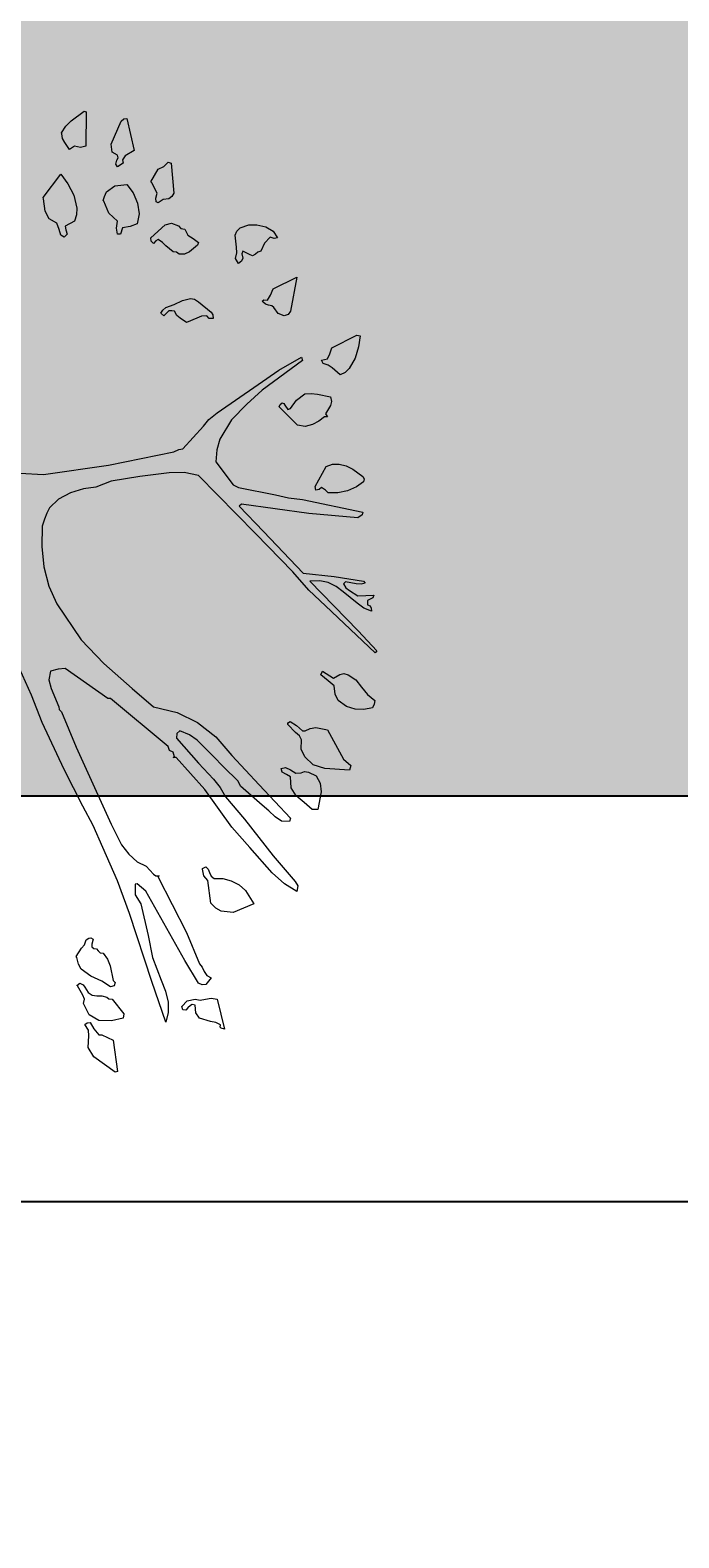
# Model space of a CAD drawing. Units: inches. Extents: x 84 to 1044, y -280 to 906.
# Tile 42 of 105: x 941 to 955, y -129 to -96. Entities that reach past the tile are written whole.
import ezdxf

# ---------------------------------------------------------------- set-up
doc = ezdxf.new("R2010")
doc.units = ezdxf.units.IN
for name, color, linetype, lineweight in [('A-ANNO-DIMS', 2, 'Continuous', 18), ('C-PROP', 7, 'Continuous', 25), ('L-PLNT', 114, 'Continuous', 15)]:
    doc.layers.add(name, color=color, linetype=linetype, lineweight=lineweight)
doc.layers.add('L-PLNT-PATT', color=9, linetype='Continuous', lineweight=9, true_color=0xafd9aa)
doc.styles.get("Standard").update_dxf_attribs({"font": 'arial.ttf'})
doc.dimstyles.get("Standard").update_dxf_attribs({"dimtxt": 0.18, "dimasz": 0.18, "dimexe": 0.18, "dimexo": 0.0625, "dimgap": 0.09, "dimtad": 0, "dimtih": 1, "dimtoh": 1, "dimdec": 4, "dimzin": 0, "dimdsep": 46, "dimtxsty": 'Standard', "dimcen": 0.09, "dimadec": 0, "dimazin": 0, "dimtfac": 1, "dimtdec": 4, "dimtofl": 0, "dimtmove": 0, "dimatfit": 3, "dimfxl": 1, "dimtolj": 1, "dimtzin": 0, "dimarcsym": 0})

# ---------------------------------------------------------------- blocks, each defined once
blk = doc.blocks.new('A$C37E508DF')
for p, q in [((0.9605, 1.4257), (0.9686, 1.4334)), ((0.9686, 1.4334), (0.9875, 1.4476)), ((0.9875, 1.4476), (0.9905, 1.4467)), ((0.9905, 1.4467), (0.9896, 1.3966)), ((1.0269, 1.3996), (1.0411, 1.433)), ((1.0411, 1.433), (1.045, 1.4365)), ((1.045, 1.4365), (1.0497, 1.4369)), ((1.0497, 1.4369), (1.0604, 1.3901)), ((0.9545, 1.4159), (0.9605, 1.4257)), ((0.9549, 1.4146), (0.9545, 1.4159)), ((0.9558, 1.4077), (0.9549, 1.4146)), ((0.9592, 1.4017), (0.9558, 1.4077)), ((0.966, 1.3914), (0.9592, 1.4017)), ((0.9703, 1.3944), (0.966, 1.3914)), ((0.9733, 1.3966), (0.9703, 1.3944)), ((0.9819, 1.3944), (0.9733, 1.3966)), ((0.9896, 1.3966), (0.9819, 1.3944)), ((1.0282, 1.3876), (1.0269, 1.3996)), ((1.0359, 1.3833), (1.0282, 1.3876)), ((1.0604, 1.3901), (1.0471, 1.3824)), ((1.0334, 1.37), (1.0351, 1.376)), ((1.0359, 1.3661), (1.0334, 1.37)), ((1.0351, 1.376), (1.0368, 1.3794)), ((1.0368, 1.3794), (1.0359, 1.3833)), ((1.0441, 1.3717), (1.0359, 1.3661)), ((1.0471, 1.3824), (1.0432, 1.3764)), ((1.0432, 1.3764), (1.0441, 1.3717)), ((1.0955, 1.3631), (1.1033, 1.367)), ((1.1033, 1.367), (1.1097, 1.373)), ((1.1097, 1.373), (1.114, 1.3717)), ((1.114, 1.3717), (1.1183, 1.328)), ((0.9274, 1.3215), (0.9532, 1.3554)), ((0.9532, 1.3554), (0.9635, 1.3413)), ((1.0848, 1.3443), (1.0955, 1.3631)), ((1.0861, 1.343), (1.0848, 1.3443)), ((1.0938, 1.328), (1.0861, 1.343)), ((0.9279, 1.3194), (0.9274, 1.3215)), ((0.9635, 1.3413), (0.9721, 1.325)), ((0.9721, 1.325), (0.9768, 1.3061)), ((1.0149, 1.3172), (1.0171, 1.3232)), ((1.0171, 1.3232), (1.0197, 1.3297)), ((1.0197, 1.3297), (1.0321, 1.3387)), ((1.0321, 1.3387), (1.0497, 1.3404)), ((1.0497, 1.3404), (1.0587, 1.3284)), ((1.0587, 1.3284), (1.0651, 1.3134)), ((1.0917, 1.3207), (1.0938, 1.328)), ((1.0925, 1.3151), (1.0917, 1.3207)), ((1.1153, 1.3228), (1.111, 1.3194)), ((1.1183, 1.328), (1.1153, 1.3228)), ((0.9305, 1.3018), (0.9279, 1.3194)), ((0.9365, 1.2902), (0.9305, 1.3018)), ((0.9768, 1.3061), (0.9763, 1.2962)), ((1.0162, 1.3164), (1.0149, 1.3172)), ((1.0231, 1.2988), (1.0162, 1.3164)), ((1.0359, 1.2868), (1.0231, 1.2988)), ((1.0651, 1.3134), (1.0677, 1.2975)), ((1.0955, 1.3138), (1.0925, 1.3151)), ((1.1028, 1.3185), (1.0955, 1.3138)), ((1.111, 1.3194), (1.1028, 1.3185)), ((0.9476, 1.2842), (0.9365, 1.2902)), ((0.951, 1.2748), (0.9476, 1.2842)), ((0.9733, 1.2868), (0.9596, 1.2799)), ((0.9596, 1.2799), (0.9605, 1.2744)), ((0.9763, 1.2962), (0.9733, 1.2868)), ((1.0347, 1.2769), (1.0359, 1.2868)), ((1.0359, 1.2679), (1.0347, 1.2769)), ((1.0432, 1.2774), (1.0402, 1.2679)), ((1.0544, 1.2791), (1.0432, 1.2774)), ((1.0647, 1.2829), (1.0544, 1.2791)), ((1.0677, 1.2975), (1.0647, 1.2829)), ((1.0848, 1.2628), (1.1054, 1.2817)), ((1.1054, 1.2817), (1.1148, 1.2842)), ((1.1148, 1.2842), (1.1247, 1.2804)), ((1.1247, 1.2804), (1.1281, 1.2765)), ((1.1281, 1.2765), (1.1341, 1.2752)), ((1.21, 1.2726), (1.2147, 1.2774)), ((1.2147, 1.2774), (1.2276, 1.2817)), ((1.2276, 1.2817), (1.2392, 1.2817)), ((1.2392, 1.2817), (1.2521, 1.2787)), ((1.2521, 1.2787), (1.2632, 1.2722)), ((0.9532, 1.2666), (0.951, 1.2748)), ((0.9583, 1.2636), (0.9532, 1.2666)), ((0.9626, 1.2679), (0.9583, 1.2636)), ((0.9605, 1.2744), (0.9626, 1.2679)), ((1.0402, 1.2679), (1.0359, 1.2679)), ((1.0852, 1.2576), (1.0848, 1.2628)), ((1.0883, 1.2546), (1.0852, 1.2576)), ((1.0921, 1.2585), (1.0883, 1.2546)), ((1.0955, 1.2602), (1.0921, 1.2585)), ((1.1015, 1.2559), (1.0955, 1.2602)), ((1.1063, 1.2508), (1.1015, 1.2559)), ((1.1341, 1.2752), (1.1384, 1.2666)), ((1.1384, 1.2666), (1.1461, 1.2619)), ((1.1461, 1.2619), (1.1539, 1.2559)), ((1.1539, 1.2559), (1.1526, 1.2521)), ((1.2075, 1.2666), (1.21, 1.2726)), ((1.2096, 1.2491), (1.2075, 1.2666)), ((1.2503, 1.2551), (1.2448, 1.2431)), ((1.2585, 1.2636), (1.2503, 1.2551)), ((1.2645, 1.2615), (1.2585, 1.2636)), ((1.2632, 1.2722), (1.2692, 1.2628)), ((1.2692, 1.2628), (1.2645, 1.2615)), ((1.117, 1.2422), (1.1063, 1.2508)), ((1.1221, 1.2418), (1.117, 1.2422)), ((1.126, 1.2388), (1.1221, 1.2418)), ((1.1337, 1.2388), (1.126, 1.2388)), ((1.141, 1.2422), (1.1337, 1.2388)), ((1.1526, 1.2521), (1.141, 1.2422)), ((1.2079, 1.2323), (1.21, 1.2409)), ((1.2126, 1.2251), (1.2079, 1.2323)), ((1.21, 1.2409), (1.2096, 1.2491)), ((1.2186, 1.2332), (1.2169, 1.2285)), ((1.2186, 1.2431), (1.2173, 1.2392)), ((1.2173, 1.2392), (1.2186, 1.2332)), ((1.2285, 1.2383), (1.2186, 1.2431)), ((1.2328, 1.2366), (1.2285, 1.2383)), ((1.2371, 1.2388), (1.2328, 1.2366)), ((1.2405, 1.2418), (1.2371, 1.2388)), ((1.2448, 1.2431), (1.2405, 1.2418)), ((1.2169, 1.2285), (1.2126, 1.2251)), ((1.2589, 1.1792), (1.2628, 1.1882)), ((1.2628, 1.1882), (1.2975, 1.2053)), ((1.2975, 1.2053), (1.2885, 1.1556)), ((1.1187, 1.1655), (1.1307, 1.1714)), ((1.1307, 1.1714), (1.1423, 1.1744)), ((1.1423, 1.1744), (1.1483, 1.1732)), ((1.1483, 1.1732), (1.1539, 1.1693)), ((1.1539, 1.1693), (1.1727, 1.1543)), ((1.2469, 1.1702), (1.2495, 1.1723)), ((1.2478, 1.1693), (1.2469, 1.1702)), ((1.2516, 1.1659), (1.2478, 1.1693)), ((1.2495, 1.1723), (1.2546, 1.1719)), ((1.2546, 1.1719), (1.2589, 1.1792)), ((1.099, 1.153), (1.102, 1.1573)), ((1.1033, 1.1487), (1.099, 1.153)), ((1.102, 1.1573), (1.1063, 1.1612)), ((1.111, 1.156), (1.1033, 1.1487)), ((1.1063, 1.1612), (1.1187, 1.1655)), ((1.1153, 1.1564), (1.111, 1.156)), ((1.1191, 1.1556), (1.1153, 1.1564)), ((1.1226, 1.1492), (1.1191, 1.1556)), ((1.1273, 1.1453), (1.1226, 1.1492)), ((1.1367, 1.1393), (1.1273, 1.1453)), ((1.1517, 1.1453), (1.1367, 1.1393)), ((1.1586, 1.1483), (1.1517, 1.1453)), ((1.1663, 1.1487), (1.1586, 1.1483)), ((1.1697, 1.1449), (1.1663, 1.1487)), ((1.1757, 1.1449), (1.1697, 1.1449)), ((1.1727, 1.1543), (1.1749, 1.1504)), ((1.1749, 1.1504), (1.1757, 1.1449)), ((1.2563, 1.1646), (1.2516, 1.1659)), ((1.2611, 1.1637), (1.2563, 1.1646)), ((1.2641, 1.1612), (1.2611, 1.1637)), ((1.2701, 1.1522), (1.2641, 1.1612)), ((1.2791, 1.1487), (1.2701, 1.1522)), ((1.2851, 1.1509), (1.2791, 1.1487)), ((1.2885, 1.1556), (1.2851, 1.1509)), ((1.3455, 1.0934), (1.3485, 1.102)), ((1.3485, 1.102), (1.385, 1.1209)), ((1.3875, 1.1037), (1.3828, 1.087)), ((1.385, 1.1209), (1.3897, 1.1196)), ((1.3897, 1.1196), (1.3875, 1.1037)), ((1.3057, 1.0835), (1.2469, 1.0402)), ((1.2713, 1.0694), (1.3044, 1.0887)), ((1.3044, 1.0887), (1.3057, 1.0835)), ((1.3335, 1.0844), (1.3421, 1.0861)), ((1.3361, 1.0793), (1.3335, 1.0844)), ((1.3434, 1.0771), (1.3361, 1.0793)), ((1.3421, 1.0861), (1.3455, 1.0934)), ((1.3828, 1.087), (1.3738, 1.072)), ((1.2409, 1.0488), (1.2713, 1.0694)), ((1.349, 1.0728), (1.3434, 1.0771)), ((1.3605, 1.063), (1.349, 1.0728)), ((1.3678, 1.0664), (1.3605, 1.063)), ((1.3738, 1.072), (1.3678, 1.0664)), ((1.1813, 1.0072), (1.2409, 1.0488)), ((1.2469, 1.0402), (1.2246, 1.0201)), ((1.2971, 1.0257), (1.3091, 1.0351)), ((1.3091, 1.0351), (1.3185, 1.0355)), ((1.3185, 1.0355), (1.3275, 1.0347)), ((1.3275, 1.0347), (1.3468, 1.0308)), ((1.2246, 1.0201), (1.2023, 0.9969)), ((1.2718, 1.0162), (1.2731, 1.0197)), ((1.2984, 0.9892), (1.2718, 1.0162)), ((1.2731, 1.0197), (1.2761, 1.0218)), ((1.2761, 1.0218), (1.2786, 1.0209)), ((1.2786, 1.0209), (1.2799, 1.0184)), ((1.2799, 1.0184), (1.2842, 1.0124)), ((1.2842, 1.0124), (1.2885, 1.0136)), ((1.2885, 1.0136), (1.2971, 1.0257)), ((1.3468, 1.018), (1.3391, 1.0059)), ((1.3468, 1.0308), (1.3481, 1.0239)), ((1.3481, 1.0239), (1.3468, 1.018)), ((1.1612, 0.9879), (1.1693, 0.9974)), ((1.1693, 0.9974), (1.1813, 1.0072)), ((1.2023, 0.9969), (1.1852, 0.9691)), ((1.3202, 0.9901), (1.3095, 0.9875)), ((1.3297, 0.9952), (1.3202, 0.9901)), ((1.3378, 1.0016), (1.3297, 0.9952)), ((1.3421, 1.0016), (1.3378, 1.0016)), ((1.3391, 1.0059), (1.3421, 1.0016)), ((1.1311, 0.9549), (1.1612, 0.9879)), ((1.1852, 0.9691), (1.1809, 0.9532)), ((1.3095, 0.9875), (1.2984, 0.9892)), ((1.0227, 0.9309), (1.1183, 0.9506)), ((1.1183, 0.9506), (1.1256, 0.954)), ((1.1256, 0.954), (1.1311, 0.9549)), ((1.1809, 0.9532), (1.1796, 0.936)), ((0.9279, 0.9172), (1.0227, 0.9309)), ((1.1796, 0.936), (1.2049, 0.9022)), ((1.3241, 0.9), (1.3404, 0.9292)), ((1.3404, 0.9292), (1.3494, 0.9322)), ((1.3494, 0.9322), (1.3592, 0.9326)), ((1.3592, 0.9326), (1.3695, 0.93)), ((1.3695, 0.93), (1.3794, 0.9253)), ((1.3794, 0.9253), (1.394, 0.9146)), ((0.8936, 0.9193), (0.9279, 0.9172)), ((1.0269, 0.9077), (1.0042, 0.8987)), ((1.0685, 0.9142), (1.0269, 0.9077)), ((1.1114, 0.9198), (1.0685, 0.9142)), ((1.1333, 0.9202), (1.1114, 0.9198)), ((1.1543, 0.9159), (1.1333, 0.9202)), ((1.2371, 0.8314), (1.1543, 0.9159)), ((1.2049, 0.9022), (1.2126, 0.8983)), ((1.3948, 0.9065), (1.3846, 0.8992)), ((1.394, 0.9146), (1.3957, 0.9112)), ((1.3957, 0.9112), (1.3948, 0.9065)), ((0.9498, 0.8816), (0.9369, 0.8687)), ((0.9673, 0.8906), (0.9498, 0.8816)), ((0.9866, 0.8962), (0.9673, 0.8906)), ((1.0042, 0.8987), (0.9866, 0.8962)), ((1.2126, 0.8983), (1.2662, 0.8876)), ((1.2662, 0.8876), (1.2855, 0.8833)), ((1.2855, 0.8833), (1.3057, 0.8807)), ((1.3057, 0.8807), (1.394, 0.8623)), ((1.3254, 0.8944), (1.3241, 0.9)), ((1.3301, 0.8957), (1.3254, 0.8944)), ((1.3335, 0.8983), (1.3301, 0.8957)), ((1.3395, 0.8944), (1.3335, 0.8983)), ((1.3434, 0.8906), (1.3395, 0.8944)), ((1.3571, 0.8906), (1.3434, 0.8906)), ((1.3713, 0.8936), (1.3571, 0.8906)), ((1.3846, 0.8992), (1.3713, 0.8936)), ((0.933, 0.861), (0.9296, 0.852)), ((0.9369, 0.8687), (0.933, 0.861)), ((1.2169, 0.8743), (1.2135, 0.8713)), ((1.2135, 0.8713), (1.2491, 0.834)), ((1.3151, 0.8606), (1.2169, 0.8743)), ((1.3863, 0.8541), (1.3151, 0.8606)), ((1.3927, 0.8584), (1.3863, 0.8541)), ((1.394, 0.8623), (1.3927, 0.8584)), ((0.9262, 0.8421), (0.9257, 0.8121)), ((0.9296, 0.852), (0.9262, 0.8421)), ((1.2919, 0.7752), (1.2371, 0.8314)), ((1.2491, 0.834), (1.3069, 0.7735)), ((0.9257, 0.8121), (0.9287, 0.7825)), ((0.9287, 0.7825), (0.936, 0.7542)), ((1.3151, 0.7487), (1.2919, 0.7752)), ((1.3069, 0.7735), (1.352, 0.7684)), ((0.936, 0.7542), (0.9476, 0.7285)), ((1.3391, 0.7255), (1.3151, 0.7487)), ((1.3309, 0.7624), (1.3164, 0.7615)), ((1.3164, 0.7615), (1.3871, 0.6891)), ((1.3434, 0.7598), (1.3309, 0.7624)), ((1.355, 0.7538), (1.3434, 0.7598)), ((1.352, 0.7684), (1.3948, 0.7615)), ((1.3653, 0.7461), (1.355, 0.7538)), ((1.3687, 0.7607), (1.3657, 0.7577)), ((1.3657, 0.7577), (1.3691, 0.7521)), ((1.3841, 0.7577), (1.3687, 0.7607)), ((1.3691, 0.7521), (1.3743, 0.7482)), ((1.3743, 0.7482), (1.3863, 0.7405)), ((1.3914, 0.7572), (1.3841, 0.7577)), ((1.397, 0.759), (1.3914, 0.7572)), ((1.3948, 0.7615), (1.397, 0.759)), ((0.9476, 0.7285), (0.9828, 0.6762)), ((1.3854, 0.7294), (1.3653, 0.7461)), ((1.3953, 0.7221), (1.3854, 0.7294)), ((1.3863, 0.7405), (1.4099, 0.7414)), ((1.4086, 0.7375), (1.4004, 0.7337)), ((1.4004, 0.7337), (1.4004, 0.7272)), ((1.4004, 0.7272), (1.4047, 0.7255)), ((1.4099, 0.7414), (1.4086, 0.7375)), ((1.4116, 0.6569), (1.3391, 0.7255)), ((1.4064, 0.7178), (1.3953, 0.7221)), ((1.4047, 0.7255), (1.406, 0.7221)), ((1.406, 0.7221), (1.4064, 0.7178)), ((1.3871, 0.6891), (1.4141, 0.6599)), ((0.9828, 0.6762), (1.0162, 0.6415)), ((1.0162, 0.6415), (1.0574, 0.605)), ((1.4141, 0.6599), (1.4116, 0.6569)), ((0.9103, 0.5956), (0.8932, 0.6342)), ((0.9382, 0.6303), (0.936, 0.6179)), ((0.936, 0.6179), (0.939, 0.605)), ((0.9493, 0.6333), (0.9382, 0.6303)), ((0.9596, 0.6342), (0.9493, 0.6333)), ((1.0218, 0.5904), (0.9596, 0.6342)), ((1.3327, 0.6252), (1.3348, 0.6303)), ((1.343, 0.6162), (1.3327, 0.6252)), ((1.3348, 0.6303), (1.3511, 0.62)), ((1.352, 0.6089), (1.343, 0.6162)), ((1.3511, 0.62), (1.3601, 0.6256)), ((1.3601, 0.6256), (1.3661, 0.6269)), ((1.3661, 0.6269), (1.3725, 0.6252)), ((1.3725, 0.6252), (1.3837, 0.6175)), ((1.3837, 0.6175), (1.3918, 0.6072)), ((0.9262, 0.5557), (0.9103, 0.5956)), ((0.939, 0.605), (0.9506, 0.5784)), ((1.0574, 0.605), (1.0883, 0.5784)), ((1.3533, 0.5969), (1.352, 0.6089)), ((1.358, 0.5874), (1.3533, 0.5969)), ((1.3918, 0.6072), (1.4004, 0.5964)), ((1.4004, 0.5964), (1.4111, 0.5874)), ((0.9506, 0.5784), (0.951, 0.5746)), ((0.951, 0.5746), (0.9545, 0.5711)), ((1.0256, 0.5904), (1.0218, 0.5904)), ((1.1097, 0.5205), (1.0256, 0.5904)), ((1.0883, 0.5784), (1.123, 0.5703)), ((1.37, 0.5789), (1.358, 0.5874)), ((1.3824, 0.575), (1.37, 0.5789)), ((1.3953, 0.5746), (1.3824, 0.575)), ((1.4077, 0.5771), (1.3953, 0.5746)), ((1.4103, 0.5823), (1.4077, 0.5771)), ((1.4111, 0.5874), (1.4103, 0.5823)), ((0.9583, 0.4871), (0.9262, 0.5557)), ((0.9545, 0.5711), (0.9759, 0.5193)), ((1.123, 0.5703), (1.1526, 0.5557)), ((1.1526, 0.5557), (1.1792, 0.5347)), ((1.2842, 0.554), (1.2855, 0.5557)), ((1.2842, 0.5527), (1.2842, 0.554)), ((1.2958, 0.5407), (1.2842, 0.5527)), ((1.2855, 0.5557), (1.2876, 0.557)), ((1.2876, 0.557), (1.2971, 0.551)), ((1.2971, 0.551), (1.3057, 0.5433)), ((1.1226, 0.5394), (1.1221, 0.5325)), ((1.1221, 0.5325), (1.1539, 0.4961)), ((1.1268, 0.5433), (1.1226, 0.5394)), ((1.141, 0.5377), (1.1268, 0.5433)), ((1.1521, 0.5296), (1.141, 0.5377)), ((1.1706, 0.5111), (1.1521, 0.5296)), ((1.1792, 0.5347), (1.2027, 0.5072)), ((1.3014, 0.536), (1.2958, 0.5407)), ((1.3044, 0.53), (1.3014, 0.536)), ((1.3039, 0.5167), (1.3044, 0.53)), ((1.3057, 0.5433), (1.3099, 0.5433)), ((1.3099, 0.5433), (1.3172, 0.5467)), ((1.3172, 0.5467), (1.3254, 0.548)), ((1.3254, 0.548), (1.3421, 0.5446)), ((1.3421, 0.5446), (1.3657, 0.5021)), ((0.9759, 0.5193), (1.0269, 0.4069)), ((1.1118, 0.5145), (1.1097, 0.5205)), ((1.117, 0.5124), (1.1118, 0.5145)), ((1.1191, 0.5055), (1.117, 0.5124)), ((1.1955, 0.4858), (1.1706, 0.5111)), ((1.2027, 0.5072), (1.2426, 0.4644)), ((1.3091, 0.5055), (1.3039, 0.5167)), ((0.9853, 0.4335), (0.9583, 0.4871)), ((1.117, 0.5042), (1.1191, 0.5055)), ((1.1217, 0.5042), (1.117, 0.5042)), ((1.1633, 0.4575), (1.1217, 0.5042)), ((1.1539, 0.4961), (1.1762, 0.4729)), ((1.207, 0.4747), (1.1955, 0.4858)), ((1.2748, 0.4884), (1.2812, 0.4897)), ((1.2761, 0.4832), (1.2748, 0.4884)), ((1.2812, 0.4897), (1.2885, 0.4862)), ((1.2885, 0.4862), (1.2962, 0.4815)), ((1.3039, 0.482), (1.3087, 0.4841)), ((1.3087, 0.4841), (1.3147, 0.4832)), ((1.3215, 0.4935), (1.3091, 0.5055)), ((1.3382, 0.4884), (1.3215, 0.4935)), ((1.3743, 0.4858), (1.3382, 0.4884)), ((1.3657, 0.5021), (1.3764, 0.4927)), ((1.3764, 0.4927), (1.3743, 0.4858)), ((1.1762, 0.4729), (1.1856, 0.4605)), ((1.2122, 0.47), (1.207, 0.4747)), ((1.2156, 0.4627), (1.2122, 0.47)), ((1.2469, 0.4348), (1.2156, 0.4627)), ((1.2426, 0.4644), (1.2885, 0.4159)), ((1.2825, 0.4798), (1.2761, 0.4832)), ((1.2885, 0.4764), (1.2825, 0.4798)), ((1.2894, 0.4601), (1.2885, 0.4764)), ((1.2962, 0.4815), (1.3039, 0.482)), ((1.3147, 0.4832), (1.3258, 0.4777)), ((1.3258, 0.4777), (1.3318, 0.4669)), ((1.3318, 0.4669), (1.3331, 0.4545)), ((1.2027, 0.4026), (1.1633, 0.4575)), ((1.1856, 0.4605), (1.1933, 0.4468)), ((1.1933, 0.4468), (1.2212, 0.4146)), ((1.2967, 0.4485), (1.2894, 0.4601)), ((1.3082, 0.4386), (1.2967, 0.4485)), ((1.3331, 0.4545), (1.3284, 0.4284)), ((1.0003, 0.4052), (0.9853, 0.4335)), ((1.2568, 0.4266), (1.2469, 0.4348)), ((1.2658, 0.4176), (1.2568, 0.4266)), ((1.3198, 0.4284), (1.3082, 0.4386)), ((1.3284, 0.4284), (1.3198, 0.4284)), ((1.0145, 0.373), (1.0003, 0.4052)), ((1.0269, 0.4069), (1.0419, 0.3769)), ((1.2289, 0.373), (1.2027, 0.4026)), ((1.2212, 0.4146), (1.2628, 0.361)), ((1.2752, 0.4116), (1.2658, 0.4176)), ((1.2868, 0.4108), (1.2752, 0.4116)), ((1.2885, 0.4159), (1.2868, 0.4108)), ((1.0419, 0.3769), (1.0527, 0.3632)), ((1.0359, 0.3246), (1.0145, 0.373)), ((1.0527, 0.3632), (1.0647, 0.352)), ((1.0647, 0.352), (1.078, 0.346)), ((1.2615, 0.3362), (1.2289, 0.373)), ((1.2628, 0.361), (1.2949, 0.3233)), ((1.078, 0.346), (1.0883, 0.334)), ((1.0883, 0.334), (1.0921, 0.3319)), ((1.0921, 0.3319), (1.0968, 0.3319)), ((1.0968, 0.3319), (1.0947, 0.3306)), ((1.0947, 0.3306), (1.1367, 0.2491)), ((1.1599, 0.3426), (1.1646, 0.3447)), ((1.1599, 0.3413), (1.1599, 0.3426)), ((1.162, 0.3319), (1.1599, 0.3413)), ((1.1676, 0.325), (1.162, 0.3319)), ((1.1646, 0.3447), (1.168, 0.3417)), ((1.168, 0.3417), (1.1702, 0.3366)), ((1.1702, 0.3366), (1.1727, 0.3314)), ((1.1727, 0.3314), (1.177, 0.3276)), ((1.2795, 0.3199), (1.2615, 0.3362)), ((1.0535, 0.2766), (1.0359, 0.3246)), ((1.0647, 0.3199), (1.0617, 0.3194)), ((1.0617, 0.3194), (1.0617, 0.304)), ((1.0711, 0.3147), (1.0647, 0.3199)), ((1.0775, 0.3092), (1.0711, 0.3147)), ((1.1341, 0.2084), (1.0775, 0.3092)), ((1.1719, 0.292), (1.1676, 0.325)), ((1.177, 0.3276), (1.1895, 0.3276)), ((1.1895, 0.3276), (1.2019, 0.3246)), ((1.2019, 0.3246), (1.2135, 0.3186)), ((1.2135, 0.3186), (1.2225, 0.3104)), ((1.2225, 0.3104), (1.2349, 0.2911)), ((1.2975, 0.3087), (1.2795, 0.3199)), ((1.2949, 0.3233), (1.2988, 0.3173)), ((1.2988, 0.3173), (1.2975, 0.3087)), ((1.0617, 0.304), (1.0698, 0.2911)), ((1.0698, 0.2911), (1.0805, 0.2448)), ((1.1792, 0.2847), (1.1719, 0.292)), ((1.2349, 0.2911), (1.2049, 0.2783)), ((1.0861, 0.1775), (1.0535, 0.2766)), ((1.1873, 0.28), (1.1792, 0.2847)), ((1.2049, 0.2783), (1.1873, 0.28)), ((1.0805, 0.2448), (1.087, 0.2127)), ((1.1367, 0.2491), (1.1556, 0.2032)), ((0.9759, 0.214), (0.9836, 0.226)), ((0.9836, 0.226), (0.9879, 0.2311)), ((0.9879, 0.2311), (0.9905, 0.2384)), ((0.9905, 0.2384), (0.9943, 0.241)), ((0.9943, 0.241), (0.9973, 0.2414)), ((0.9973, 0.2414), (1.0003, 0.2393)), ((1.0003, 0.2393), (0.9986, 0.232)), ((0.9986, 0.232), (0.9986, 0.2281)), ((0.9986, 0.2281), (1.0012, 0.2255)), ((1.0012, 0.2255), (1.0051, 0.2251)), ((1.0051, 0.2251), (1.0076, 0.2225)), ((1.0076, 0.2225), (1.0106, 0.2195)), ((0.9768, 0.2127), (0.9759, 0.214)), ((0.9789, 0.2028), (0.9768, 0.2127)), ((0.9832, 0.1955), (0.9789, 0.2028)), ((1.0106, 0.2195), (1.0149, 0.2191)), ((1.0149, 0.2191), (1.0214, 0.2101)), ((1.0214, 0.2101), (1.0252, 0.2002)), ((1.0252, 0.2002), (1.0295, 0.1788)), ((1.087, 0.2127), (1.0998, 0.1797)), ((1.1543, 0.1749), (1.1341, 0.2084)), ((1.1556, 0.2032), (1.1594, 0.1985)), ((1.1594, 0.1985), (1.1624, 0.1921)), ((0.9969, 0.1852), (0.9832, 0.1955)), ((1.0132, 0.1779), (0.9969, 0.1852)), ((1.0256, 0.1698), (1.0132, 0.1779)), ((1.0295, 0.1788), (1.0325, 0.1762)), ((1.0325, 0.1762), (1.0312, 0.1711)), ((1.1063, 0.1183), (1.0861, 0.1775)), ((1.0998, 0.1797), (1.1058, 0.1634)), ((1.1624, 0.1921), (1.1663, 0.1861)), ((1.1727, 0.1827), (1.1646, 0.1732)), ((1.1663, 0.1861), (1.1727, 0.1827)), ((0.9768, 0.1719), (0.9811, 0.1749)), ((0.9776, 0.1711), (0.9768, 0.1719)), ((0.9853, 0.1578), (0.9776, 0.1711)), ((0.9811, 0.1749), (0.9858, 0.1728)), ((0.9879, 0.1518), (0.9853, 0.1578)), ((0.9858, 0.1728), (0.9884, 0.1694)), ((0.9884, 0.1694), (0.9931, 0.1616)), ((0.9931, 0.1616), (0.9991, 0.1574)), ((0.9991, 0.1574), (1.0059, 0.1565)), ((1.0059, 0.1565), (1.0132, 0.1565)), ((1.0132, 0.1565), (1.0205, 0.1548)), ((1.0205, 0.1548), (1.0235, 0.1522)), ((1.0312, 0.1711), (1.0256, 0.1698)), ((1.1058, 0.1634), (1.1097, 0.1475)), ((1.1594, 0.1728), (1.1543, 0.1749)), ((1.1646, 0.1732), (1.1594, 0.1728)), ((0.9866, 0.1453), (0.9879, 0.1518)), ((0.9948, 0.1291), (0.9866, 0.1453)), ((1.0235, 0.1522), (1.0282, 0.1518)), ((1.0282, 0.1518), (1.0454, 0.1303)), ((1.1101, 0.1325), (1.1063, 0.1183)), ((1.1097, 0.1475), (1.1101, 0.1325)), ((1.1298, 0.1411), (1.1376, 0.1492)), ((1.1311, 0.1364), (1.1298, 0.1411)), ((1.1354, 0.1359), (1.1311, 0.1364)), ((1.1384, 0.1389), (1.1354, 0.1359)), ((1.1376, 0.1492), (1.1491, 0.1518)), ((1.1423, 0.1423), (1.1384, 0.1389)), ((1.1449, 0.1441), (1.1423, 0.1423)), ((1.1491, 0.1428), (1.1449, 0.1441)), ((1.1491, 0.1518), (1.1564, 0.1505)), ((1.1504, 0.132), (1.1491, 0.1428)), ((1.1556, 0.1239), (1.1504, 0.132)), ((1.1564, 0.1505), (1.1642, 0.1518)), ((1.1642, 0.1518), (1.1727, 0.1531)), ((1.1727, 0.1531), (1.1813, 0.1518)), ((1.1813, 0.1518), (1.192, 0.108)), ((0.9884, 0.1149), (0.9918, 0.117)), ((0.9935, 0.1063), (0.9884, 0.1149)), ((0.9918, 0.117), (0.9961, 0.1175)), ((1.0089, 0.1205), (0.9948, 0.1291)), ((0.9961, 0.1175), (1.0016, 0.1085)), ((1.0274, 0.12), (1.0089, 0.1205)), ((1.0441, 0.1239), (1.0274, 0.12)), ((1.0454, 0.1303), (1.0441, 0.1239)), ((1.1714, 0.1192), (1.1556, 0.1239)), ((1.1792, 0.1179), (1.1714, 0.1192)), ((1.186, 0.1145), (1.1792, 0.1179)), ((1.1856, 0.111), (1.186, 0.1145)), ((1.1873, 0.1093), (1.1856, 0.111)), ((0.9931, 0.081), (0.9943, 0.0982)), ((0.9943, 0.0982), (0.9935, 0.1063)), ((1.0016, 0.1085), (1.0089, 0.0999)), ((1.0089, 0.0999), (1.0132, 0.0999)), ((1.0132, 0.0999), (1.0295, 0.0917)), ((1.0295, 0.0917), (1.0359, 0.0463)), ((1.192, 0.108), (1.1873, 0.1093)), ((1.0012, 0.0677), (0.9931, 0.081)), ((1.0325, 0.0454), (1.0012, 0.0677)), ((1.0359, 0.0463), (1.0325, 0.0454))]:
    blk.add_line(p, q)
blk = doc.blocks.new('*D60')
at = {"layer": 'A-ANNO-DIMS', "color": 0, "lineweight": -2, "transparency": 16777216}
for p, q in [((134.179, -121.942), (134.179, -180.64)), ((992.074, -121.942), (992.074, -180.64)), ((134.359, -180.46), (562.733, -180.46)), ((991.894, -180.46), (563.521, -180.46))]:
    blk.add_line(p, q, dxfattribs=at)
at = {"layer": 'A-ANNO-DIMS', "color": 0, "transparency": 16777216}
for points in [[(134.359, -180.43), (134.359, -180.49), (134.179, -180.46)], [(991.894, -180.43), (991.894, -180.49), (992.074, -180.46)]]:
    blk.add_solid(points, dxfattribs=at)
at = {"layer": 'Defpoints', "color": 0, "transparency": 16777216}
for p in [(134.179, -121.88), (992.074, -121.88), (992.074, -180.46)]:
    blk.add_point(p, dxfattribs=at)
at = {"layer": 'A-ANNO-DIMS', "color": 0, "transparency": 16777216, "insert": (563.127, -180.46), "char_height": 0.18, "attachment_point": 5}
blk.add_mtext('\\A1;857.9', dxfattribs=at)

msp = doc.modelspace()

# ---------------------------------------------------------------- hatches: boundary and pattern name
at = {"layer": 'L-PLNT-PATT', "transparency": 33554597}
h = msp.add_hatch(color=256, dxfattribs=at)
h.dxf.hatch_style = 1
h.paths.add_polyline_path([(791.074, 31.12), (791.074, 91.12), (743.074, 91.12), (674.074, 91.12), (674.074, 31.12), (650.074, 31.12), (650.074, -112.88), (983.074, -112.88), (983.074, -64.88), (791.074, -64.88)])

# ---------------------------------------------------------------- linework, layer by layer
at = {"layer": 'C-PROP'}
for points in [[(143.179, -121.88), (134.179, -121.88), (134.179, 856.12), (992.074, 856.12), (992.074, -121.88), (624.574, -121.88)], [(143.179, -112.88), (143.179, 847.12), (983.074, 847.12), (983.074, -112.88), (624.574, -112.88)]]:
    msp.add_lwpolyline(points, dxfattribs=at)

# ---------------------------------------------------------------- block references
at = {"layer": 'L-PLNT', "xscale": 15.19586232982809, "yscale": 15.19586232982809, "zscale": 15.19586232982809}
msp.add_blockref('A$C37E508DF', (926.909, -119.69), dxfattribs=at)

# ---------------------------------------------------------------- dimensions: what is measured, and where the dimension line sits
at = {"layer": 'A-ANNO-DIMS'}
dim = msp.add_linear_dim(base=(992.074, -180.46), p1=(134.179, -121.88), p2=(992.074, -121.88), dimstyle='Standard', override={"dimdec": 1, "dimlfac": 1, "dimrnd": 0, "dimzin": 0, "dimdsep": 46, "dimlunit": 2}, dxfattribs=at)
dim.commit()
dim.dimension.update_dxf_attribs({"geometry": '*D60', "text_midpoint": (563.127, -180.46)})

doc.saveas('drawing.dxf')
